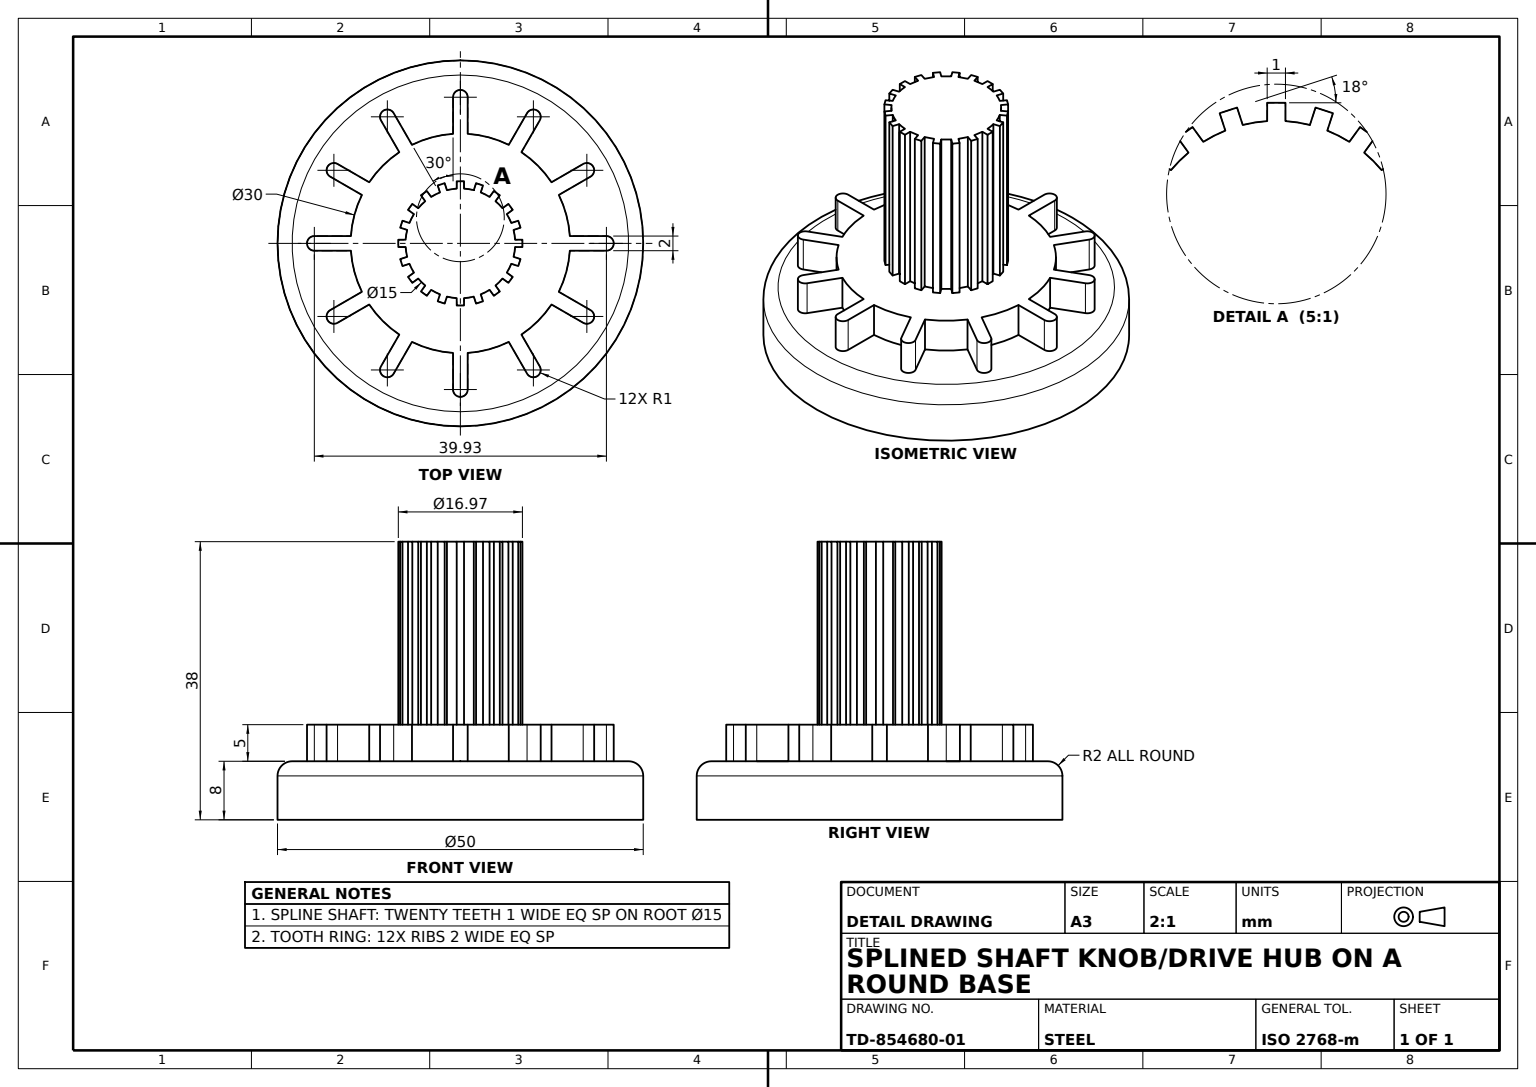
SolidWorks part; units mm, degrees
material "Plain Carbon Steel"
ref_plane "Front Plane" through (0, 0, 0) normal (0, 0, 1) x (1, 0, 0)
ref_plane "Top Plane" through (0, 0, 0) normal (0, 1, 0) x (1, 0, 0)
ref_plane "Right Plane" through (0, 0, 0) normal (1, 0, 0) x (0, 0, -1)
sketch "Base Disc Sketch" plane through (0, 0, 0) normal (0, 1, 0) x (1, 0, 0)
  circle A0 centre (0, 0) radius 25
  dimension "D1" = 50
extrude "Base Disc Ø50" add sketch "Base Disc Sketch" along normal blind 8
sketch "Tooth Ring Sketch" plane through (0, 8, 0) normal (0, 1, 0) x (1, 0, 0)
  line L0 (8.3493, 12.4615) -> (10.8493, 16.7916)
  line L2 (-1, 14.9666) -> (-1, 19.9666)
  line L4 (1, 14.9666) -> (1, 19.9666)
  line L5 (6.6173, 13.4615) -> (9.1173, 17.7916)
  line L6 (13.4615, 6.6173) -> (17.7916, 9.1173)
  line L7 (12.4615, 8.3493) -> (16.7916, 10.8493)
  line L8 (14.9666, -1) -> (19.9666, -1)
  line L9 (14.9666, 1) -> (19.9666, 1)
  line L10 (12.4615, -8.3493) -> (16.7916, -10.8493)
  line L11 (13.4615, -6.6173) -> (17.7916, -9.1173)
  line L12 (6.6173, -13.4615) -> (9.1173, -17.7916)
  line L13 (8.3493, -12.4615) -> (10.8493, -16.7916)
  line L14 (-1, -14.9666) -> (-1, -19.9666)
  line L15 (1, -14.9666) -> (1, -19.9666)
  line L16 (-8.3493, -12.4615) -> (-10.8493, -16.7916)
  line L17 (-6.6173, -13.4615) -> (-9.1173, -17.7916)
  line L18 (-13.4615, -6.6173) -> (-17.7916, -9.1173)
  line L19 (-12.4615, -8.3493) -> (-16.7916, -10.8493)
  line L20 (-14.9666, 1) -> (-19.9666, 1)
  line L21 (-14.9666, -1) -> (-19.9666, -1)
  line L22 (-12.4615, 8.3493) -> (-16.7916, 10.8493)
  line L23 (-13.4615, 6.6173) -> (-17.7916, 9.1173)
  line L24 (-6.6173, 13.4615) -> (-9.1173, 17.7916)
  line L25 (-8.3493, 12.4615) -> (-10.8493, 16.7916)
  arc A0 (-1, 14.9666) -> (-6.6173, 13.4615) centre (0, 0) ccw
  arc A1 (1, 19.9666) -> (-1, 19.9666) centre (0, 19.9666) ccw
  arc A2 (10.8493, 16.7916) -> (9.1173, 17.7916) centre (9.9833, 17.2916) ccw
  arc A3 (17.7916, 9.1173) -> (16.7916, 10.8493) centre (17.2916, 9.9833) ccw
  arc A4 (19.9666, -1) -> (19.9666, 1) centre (19.9666, 0) ccw
  arc A5 (16.7916, -10.8493) -> (17.7916, -9.1173) centre (17.2916, -9.9833) ccw
  arc A6 (9.1173, -17.7916) -> (10.8493, -16.7916) centre (9.9833, -17.2916) ccw
  arc A7 (-1, -19.9666) -> (1, -19.9666) centre (0, -19.9666) ccw
  arc A8 (-10.8493, -16.7916) -> (-9.1173, -17.7916) centre (-9.9833, -17.2916) ccw
  arc A9 (-17.7916, -9.1173) -> (-16.7916, -10.8493) centre (-17.2916, -9.9833) ccw
  arc A10 (-19.9666, 1) -> (-19.9666, -1) centre (-19.9666, 0) ccw
  arc A11 (-16.7916, 10.8493) -> (-17.7916, 9.1173) centre (-17.2916, 9.9833) ccw
  arc A12 (-9.1173, 17.7916) -> (-10.8493, 16.7916) centre (-9.9833, 17.2916) ccw
  arc A13 (-8.3493, 12.4615) -> (-12.4615, 8.3493) centre (0, 0) ccw
  arc A14 (-13.4615, 6.6173) -> (-14.9666, 1) centre (0, 0) ccw
  arc A15 (-14.9666, -1) -> (-13.4615, -6.6173) centre (0, 0) ccw
  arc A16 (-12.4615, -8.3493) -> (-8.3493, -12.4615) centre (0, 0) ccw
  arc A17 (-6.6173, -13.4615) -> (-1, -14.9666) centre (0, 0) ccw
  arc A18 (1, -14.9666) -> (6.6173, -13.4615) centre (0, 0) ccw
  arc A19 (8.3493, -12.4615) -> (12.4615, -8.3493) centre (0, 0) ccw
  arc A20 (13.4615, -6.6173) -> (14.9666, -1) centre (0, 0) ccw
  arc A21 (14.9666, 1) -> (13.4615, 6.6173) centre (0, 0) ccw
  arc A22 (12.4615, 8.3493) -> (8.3493, 12.4615) centre (0, 0) ccw
  arc A23 (6.6173, 13.4615) -> (1, 14.9666) centre (0, 0) ccw
  dimension "D1" = 30
  dimension "D5" = 1
  dimension "D2" = 1
  dimension "D3" = 2
  dimension "D4" = 5
  dimension "D8" = 4.3301
  dimension "D7" = 12
extrude "Tooth Ring 12T Ø30" add sketch "Tooth Ring Sketch" along normal blind 5
sketch "Spline Shaft Sketch" plane through (0, 13, 0) normal (0, 1, 0) x (1, 0, 0)
  line L0 (1.8369, 7.2716) -> (2.146, 8.2226)
  line L2 (-0.5, 7.4833) -> (-0.5, 8.4833)
  line L3 (-0.5, 8.4833) -> (0.5, 8.4833)
  line L4 (0.5, 7.4833) -> (0.5, 8.4833)
  line L5 (2.146, 8.2226) -> (3.097, 7.9136)
  line L6 (2.788, 6.9625) -> (3.097, 7.9136)
  line L7 (3.9941, 6.348) -> (4.5819, 7.157)
  line L8 (4.5819, 7.157) -> (5.3909, 6.5693)
  line L9 (4.8031, 5.7602) -> (5.3909, 6.5693)
  line L10 (5.7602, 4.8031) -> (6.5693, 5.3909)
  line L11 (6.5693, 5.3909) -> (7.157, 4.5819)
  line L12 (6.348, 3.9941) -> (7.157, 4.5819)
  line L13 (6.9625, 2.788) -> (7.9136, 3.097)
  line L14 (7.9136, 3.097) -> (8.2226, 2.146)
  line L15 (7.2716, 1.8369) -> (8.2226, 2.146)
  line L16 (7.4833, 0.5) -> (8.4833, 0.5)
  line L17 (8.4833, 0.5) -> (8.4833, -0.5)
  line L18 (7.4833, -0.5) -> (8.4833, -0.5)
  line L19 (7.2716, -1.8369) -> (8.2226, -2.146)
  line L20 (8.2226, -2.146) -> (7.9136, -3.097)
  line L21 (6.9625, -2.788) -> (7.9136, -3.097)
  line L22 (6.348, -3.9941) -> (7.157, -4.5819)
  line L23 (7.157, -4.5819) -> (6.5693, -5.3909)
  line L24 (5.7602, -4.8031) -> (6.5693, -5.3909)
  line L25 (4.8031, -5.7602) -> (5.3909, -6.5693)
  line L26 (5.3909, -6.5693) -> (4.5819, -7.157)
  line L27 (3.9941, -6.348) -> (4.5819, -7.157)
  line L28 (2.788, -6.9625) -> (3.097, -7.9136)
  line L29 (3.097, -7.9136) -> (2.146, -8.2226)
  line L30 (1.8369, -7.2716) -> (2.146, -8.2226)
  line L31 (0.5, -7.4833) -> (0.5, -8.4833)
  line L32 (0.5, -8.4833) -> (-0.5, -8.4833)
  line L33 (-0.5, -7.4833) -> (-0.5, -8.4833)
  line L34 (-1.8369, -7.2716) -> (-2.146, -8.2226)
  line L35 (-2.146, -8.2226) -> (-3.097, -7.9136)
  line L36 (-2.788, -6.9625) -> (-3.097, -7.9136)
  line L37 (-3.9941, -6.348) -> (-4.5819, -7.157)
  line L38 (-4.5819, -7.157) -> (-5.3909, -6.5693)
  line L39 (-4.8031, -5.7602) -> (-5.3909, -6.5693)
  line L40 (-5.7602, -4.8031) -> (-6.5693, -5.3909)
  line L41 (-6.5693, -5.3909) -> (-7.157, -4.5819)
  line L42 (-6.348, -3.9941) -> (-7.157, -4.5819)
  line L43 (-6.9625, -2.788) -> (-7.9136, -3.097)
  line L44 (-7.9136, -3.097) -> (-8.2226, -2.146)
  line L45 (-7.2716, -1.8369) -> (-8.2226, -2.146)
  line L46 (-7.4833, -0.5) -> (-8.4833, -0.5)
  line L47 (-8.4833, -0.5) -> (-8.4833, 0.5)
  line L48 (-7.4833, 0.5) -> (-8.4833, 0.5)
  line L49 (-7.2716, 1.8369) -> (-8.2226, 2.146)
  line L50 (-8.2226, 2.146) -> (-7.9136, 3.097)
  line L51 (-6.9625, 2.788) -> (-7.9136, 3.097)
  line L52 (-6.348, 3.9941) -> (-7.157, 4.5819)
  line L53 (-7.157, 4.5819) -> (-6.5693, 5.3909)
  line L54 (-5.7602, 4.8031) -> (-6.5693, 5.3909)
  line L55 (-4.8031, 5.7602) -> (-5.3909, 6.5693)
  line L56 (-5.3909, 6.5693) -> (-4.5819, 7.157)
  line L57 (-3.9941, 6.348) -> (-4.5819, 7.157)
  line L58 (-2.788, 6.9625) -> (-3.097, 7.9136)
  line L59 (-3.097, 7.9136) -> (-2.146, 8.2226)
  line L60 (-1.8369, 7.2716) -> (-2.146, 8.2226)
  arc A0 (-0.5, 7.4833) -> (-1.8369, 7.2716) centre (0, 0) ccw
  arc A1 (1.8369, 7.2716) -> (0.5, 7.4833) centre (0, 0) ccw
  arc A2 (3.9941, 6.348) -> (2.788, 6.9625) centre (0, 0) ccw
  arc A3 (5.7602, 4.8031) -> (4.8031, 5.7602) centre (0, 0) ccw
  arc A4 (6.9625, 2.788) -> (6.348, 3.9941) centre (0, 0) ccw
  arc A5 (7.4833, 0.5) -> (7.2716, 1.8369) centre (0, 0) ccw
  arc A6 (7.2716, -1.8369) -> (7.4833, -0.5) centre (0, 0) ccw
  arc A7 (6.348, -3.9941) -> (6.9625, -2.788) centre (0, 0) ccw
  arc A8 (4.8031, -5.7602) -> (5.7602, -4.8031) centre (0, 0) ccw
  arc A9 (2.788, -6.9625) -> (3.9941, -6.348) centre (0, 0) ccw
  arc A10 (0.5, -7.4833) -> (1.8369, -7.2716) centre (0, 0) ccw
  arc A11 (-1.8369, -7.2716) -> (-0.5, -7.4833) centre (0, 0) ccw
  arc A12 (-3.9941, -6.348) -> (-2.788, -6.9625) centre (0, 0) ccw
  arc A13 (-5.7602, -4.8031) -> (-4.8031, -5.7602) centre (0, 0) ccw
  arc A14 (-6.9625, -2.788) -> (-6.348, -3.9941) centre (0, 0) ccw
  arc A15 (-7.4833, -0.5) -> (-7.2716, -1.8369) centre (0, 0) ccw
  arc A16 (-7.2716, 1.8369) -> (-7.4833, 0.5) centre (0, 0) ccw
  arc A17 (-6.348, 3.9941) -> (-6.9625, 2.788) centre (0, 0) ccw
  arc A18 (-2.788, 6.9625) -> (-3.9941, 6.348) centre (0, 0) ccw
  arc A19 (-4.8031, 5.7602) -> (-5.7602, 4.8031) centre (0, 0) ccw
  dimension "D1" = 15
  dimension "D2" = 0.5
  dimension "D3" = 1
  dimension "D4" = 1
  dimension "D5" = 20
extrude "Spline Shaft 20T Ø15" add sketch "Spline Shaft Sketch" along normal blind 25
fillet "Base Edge Fillet R2" radius 2 1 edges at (0, 8, 25)
